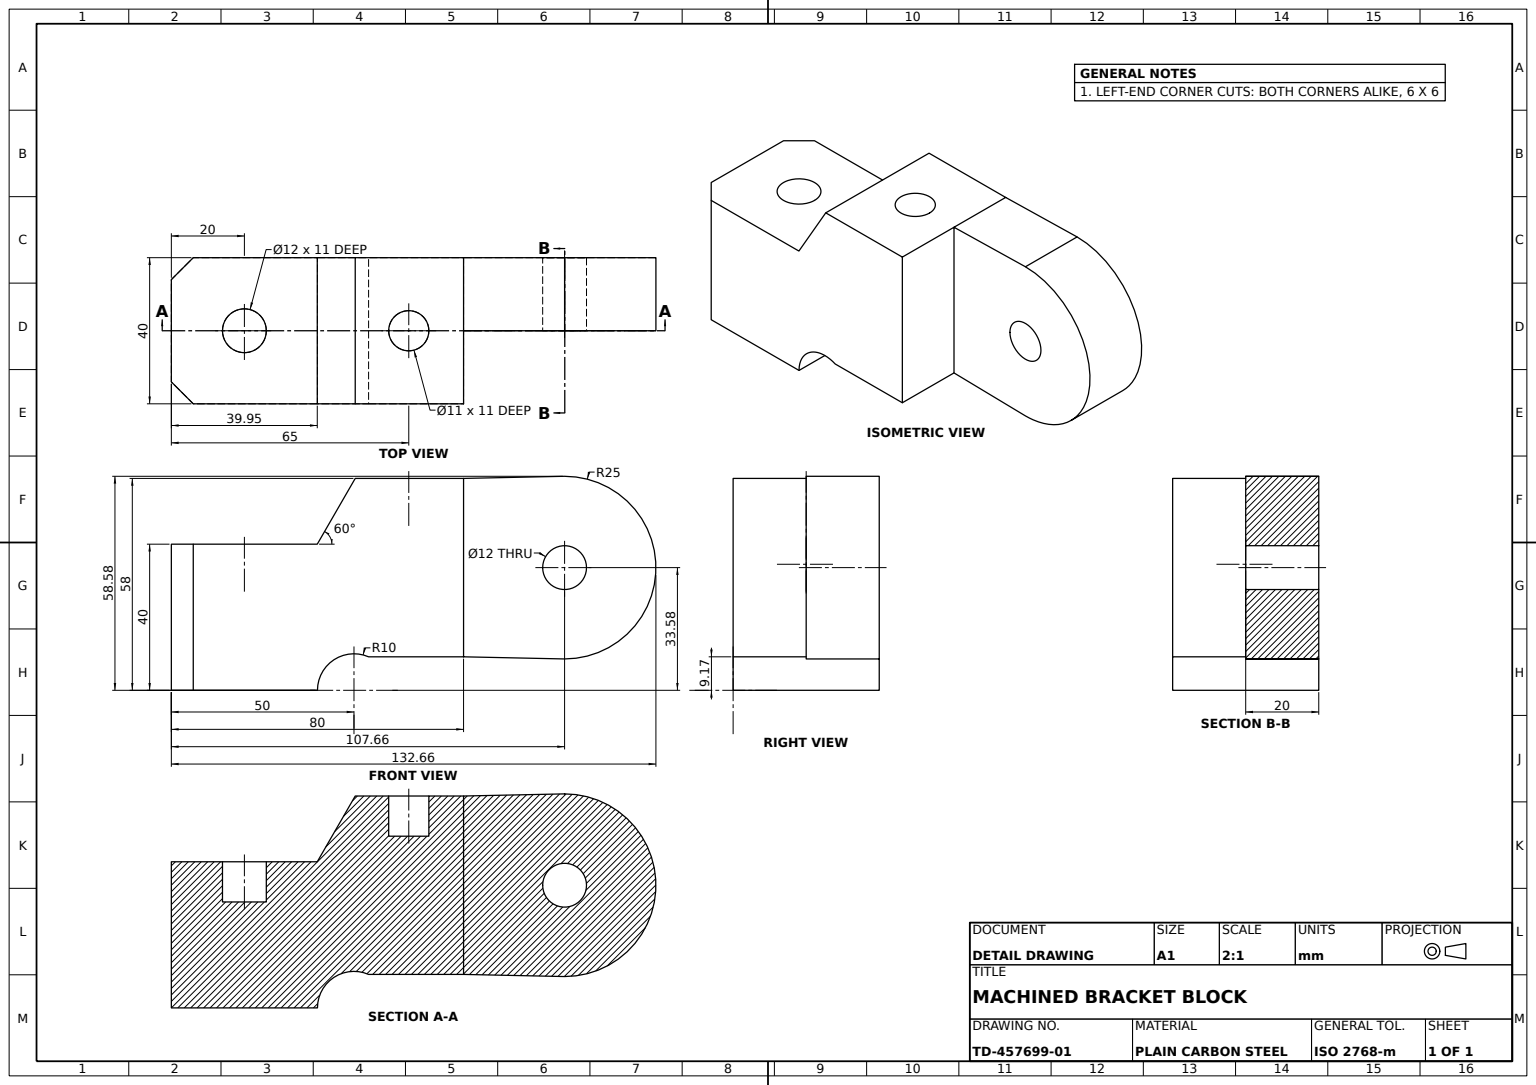
from build123d import *

# Parameters (mm, degrees)
HOUSING_BODY_DEPTH       = 20
CORNER_CUT_A_6X6_DEPTH   = 101.816665289
CORNER_CUT_B_6X6_DEPTH   = 101.816665289
STEP_HOLE_SKETCH_R       = 6
STEP_HOLE_CUT_DEPTH      = 11
SECOND_STEP_CUT_SKETCH_R = 5.5
SECOND_STEP_CUT_DEPTH    = 11
EYE_LUG_DEPTH            = 20
EYE_BORE_SKETCH_R        = 6
EYE_BORE_12_DEPTH        = 147.389505053


with BuildPart() as part:
    # Housing Profile Sketch → Housing Body (new, symmetric)
    with BuildSketch(Plane(origin=(0, 0, 0), x_dir=(0, 0, -1), z_dir=(1, 0, 0))):
        with BuildLine():
            Line((0, 0), (40, 0))
            ThreePointArc((40, 0), (44.522774425, 8.366600265), (54, 9.16515139))
            Line((54, 9.16515139), (80, 9.16515139))
            Line((80, 9.16515139), (80, 58))
            Line((80, 58), (50.341394733, 58))
            Line((50.341394733, 58), (39.949089887, 40))
            Line((39.949089887, 40), (0, 40))
            Line((0, 40), (0, 0))
        make_face()
    extrude(amount=HOUSING_BODY_DEPTH, both=True)

    # Corner Cut A Sketch → Corner Cut A 6x6 (cut, through all)
    with BuildSketch(Plane.XZ):
        Polygon((14, 0), (20, -6), (20, 0), align=None)
    extrude(amount=-CORNER_CUT_A_6X6_DEPTH, mode=Mode.SUBTRACT)

    # Corner Cut B Sketch → Corner Cut B 6x6 (cut, through all)
    with BuildSketch(Plane.XZ):
        Polygon((-20, 0), (-20, -6), (-14, 0), align=None)
    extrude(amount=-CORNER_CUT_B_6X6_DEPTH, mode=Mode.SUBTRACT)

    # Step Hole Sketch → Step Hole Cut (cut)
    with BuildSketch(Plane(origin=(0, 40, 0), x_dir=(1, 0, 0), z_dir=(0, 1, 0))):
        with Locations(Location((0, 20, 0), (0, 0, 270))):
            Circle(STEP_HOLE_SKETCH_R)
    extrude(amount=-STEP_HOLE_CUT_DEPTH, mode=Mode.SUBTRACT)

    # Second Step Cut Sketch → Second Step Cut (cut)
    with BuildSketch(Plane(origin=(0, 58, 0), x_dir=(1, 0, 0), z_dir=(0, 1, 0))):
        with Locations(Location((0, 65, 0), (0, 0, 270))):
            Circle(SECOND_STEP_CUT_SKETCH_R)
    extrude(amount=-SECOND_STEP_CUT_DEPTH, mode=Mode.SUBTRACT)

    # Eye Lug Sketch → Eye Lug (add)
    with BuildSketch(Plane.ZY.offset(20)):
        with BuildLine():
            Line((-107.657336829, 58.582575695), (-80, 58))
            Line((-80, 58), (-80, 9.16515139))
            Line((-80, 9.16515139), (-107.657336829, 8.582575695))
            ThreePointArc((-107.657336829, 8.582575695), (-132.657336829, 33.582575695), (-107.657336829, 58.582575695))
        make_face()
    extrude(amount=-EYE_LUG_DEPTH)

    # Eye Bore Sketch → Eye Bore Ø12 (cut, through all)
    with BuildSketch(Plane(origin=(0, 0, 0), x_dir=(0, 0, -1), z_dir=(1, 0, 0))):
        with Locations((107.657336829, 33.582575695)):
            Circle(EYE_BORE_SKETCH_R)
    extrude(amount=-EYE_BORE_12_DEPTH, mode=Mode.SUBTRACT)


solid = part.part
